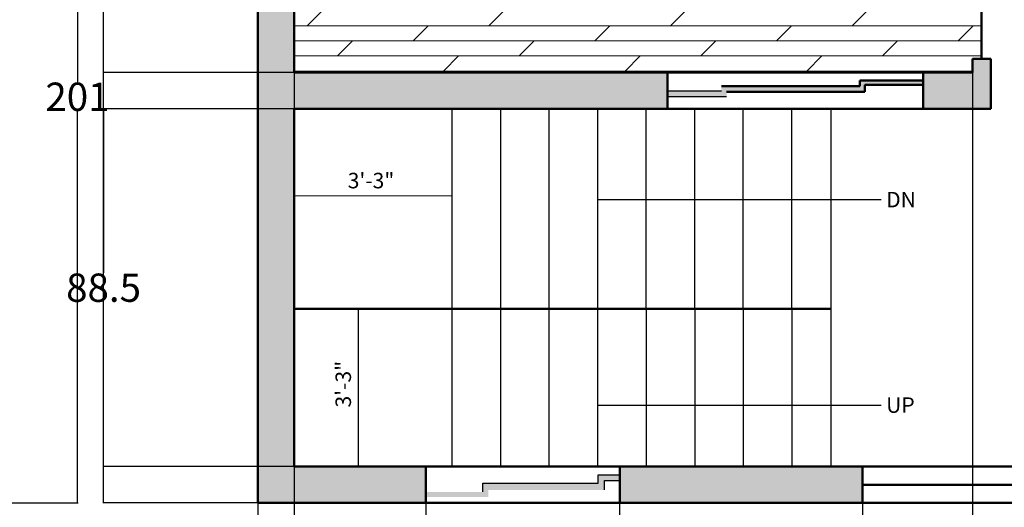
# Model space of a CAD drawing. Units: inches. Extents: x 1381 to 2246, y 1317 to 2168.
# Tile 10 of 15: x 1804 to 2048, y 1471 to 1591. Entities that reach past the tile are written whole.
import ezdxf

# ---------------------------------------------------------------- set-up
doc = ezdxf.new("R2010")
doc.units = ezdxf.units.IN
doc.header["$MEASUREMENT"] = 0
for name, color, linetype, lineweight in [('A-ANNO-DIMS', 2, 'Continuous', 18), ('A-ANNO-TEXT', 7, 'Continuous', 18), ('A-FLOR-PATT', 252, 'Continuous', 13), ('A-FLOR-STRS', 3, 'Continuous', 25), ('A-GLAZ', 4, 'Continuous', 25), ('A-WALL', 7, 'Continuous', 50), ('A-WALL-PATT', 8, 'Continuous', 13)]:
    doc.layers.add(name, color=color, linetype=linetype, lineweight=lineweight)
doc.styles.get("Standard").update_dxf_attribs({"font": 'arial.ttf'})
doc.dimstyles.get("Standard").update_dxf_attribs({"dimtxt": 7, "dimasz": 0.18, "dimexe": 0.18, "dimexo": 0.0625, "dimgap": 0.09, "dimtad": 0, "dimtih": 1, "dimtoh": 1, "dimdec": 1, "dimzin": 0, "dimdsep": 46, "dimlunit": 3, "dimtxsty": 'Standard', "dimcen": 0.09, "dimadec": 0, "dimazin": 0, "dimtfac": 1, "dimtdec": 1, "dimtofl": 0, "dimtmove": 0, "dimatfit": 3, "dimfxl": 1, "dimtolj": 1, "dimtzin": 0, "dimarcsym": 0})

# ---------------------------------------------------------------- blocks, each defined once
blk = doc.blocks.new('*D60')
at = {"layer": 'A-ANNO-DIMS', "color": 0, "lineweight": -2, "transparency": 16777216}
for p, q in [((1737.61, 1672.92), (1818.27, 1672.92)), ((1818.09, 1672.74), (1818.09, 1576.08)), ((1818.09, 1472.1), (1818.09, 1568.75)), ((1737.61, 1471.92), (1818.27, 1471.92))]:
    blk.add_line(p, q, dxfattribs=at)
at = {"layer": 'A-ANNO-DIMS', "color": 0, "transparency": 16777216}
for points in [[(1818.06, 1672.74), (1818.12, 1672.74), (1818.09, 1672.92)], [(1818.06, 1472.1), (1818.12, 1472.1), (1818.09, 1471.92)]]:
    blk.add_solid(points, dxfattribs=at)
at = {"layer": 'Defpoints', "color": 0, "transparency": 16777216}
for p in [(1737.55, 1672.92), (1818.09, 1672.92), (1737.55, 1471.92)]:
    blk.add_point(p, dxfattribs=at)
at = {"layer": 'A-ANNO-DIMS', "color": 0, "transparency": 16777216, "insert": (1818.09, 1572.42), "char_height": 7, "attachment_point": 5}
blk.add_mtext('\\A1;201', dxfattribs=at)
blk = doc.blocks.new('*D75')
at = {"layer": 'A-ANNO-DIMS', "color": 0, "lineweight": -2, "transparency": 16777216}
for p, q in [((1862.81, 1471.85), (1862.81, 1384.36)), ((2162.31, 1471.85), (2162.31, 1384.36)), ((1862.99, 1384.54), (2000.57, 1384.54)), ((2162.13, 1384.54), (2024.54, 1384.54))]:
    blk.add_line(p, q, dxfattribs=at)
at = {"layer": 'A-ANNO-DIMS', "color": 0, "transparency": 16777216}
for points in [[(1862.99, 1384.57), (1862.99, 1384.51), (1862.81, 1384.54)], [(2162.13, 1384.57), (2162.13, 1384.51), (2162.31, 1384.54)]]:
    blk.add_solid(points, dxfattribs=at)
at = {"layer": 'Defpoints', "color": 0, "transparency": 16777216}
for p in [(1862.81, 1471.92), (2162.31, 1471.92), (2162.31, 1384.54)]:
    blk.add_point(p, dxfattribs=at)
at = {"layer": 'A-ANNO-DIMS', "color": 0, "transparency": 16777216, "insert": (2012.56, 1384.54), "char_height": 7, "attachment_point": 5}
blk.add_mtext('\\A1;299.5', dxfattribs=at)
blk = doc.blocks.new('*D76')
at = {"layer": 'A-ANNO-DIMS', "color": 0, "lineweight": -2, "transparency": 16777216}
for p, q in [((1862.74, 2092.92), (1824.38, 2092.92)), ((1824.56, 2092.74), (1824.56, 1786.08)), ((1824.56, 1472.1), (1824.56, 1778.75)), ((1862.74, 1471.92), (1824.38, 1471.92))]:
    blk.add_line(p, q, dxfattribs=at)
at = {"layer": 'A-ANNO-DIMS', "color": 0, "transparency": 16777216}
for points in [[(1824.53, 2092.74), (1824.59, 2092.74), (1824.56, 2092.92)], [(1824.53, 1472.1), (1824.59, 1472.1), (1824.56, 1471.92)]]:
    blk.add_solid(points, dxfattribs=at)
at = {"layer": 'Defpoints', "color": 0, "transparency": 16777216}
for p in [(1824.56, 2092.92), (1862.81, 2092.92), (1862.81, 1471.92)]:
    blk.add_point(p, dxfattribs=at)
at = {"layer": 'A-ANNO-DIMS', "color": 0, "transparency": 16777216, "insert": (1824.56, 1782.42), "char_height": 7, "attachment_point": 5}
blk.add_mtext('\\A1;621', dxfattribs=at)
blk = doc.blocks.new('*D80')
at = {"layer": 'A-ANNO-DIMS', "color": 0, "lineweight": -2, "transparency": 16777216}
for p, q in [((1871.74, 1569.42), (1824.38, 1569.42)), ((1824.56, 1569.24), (1824.56, 1528.83)), ((1824.56, 1481.1), (1824.56, 1521.5)), ((1871.74, 1480.92), (1824.38, 1480.92))]:
    blk.add_line(p, q, dxfattribs=at)
at = {"layer": 'A-ANNO-DIMS', "color": 0, "transparency": 16777216}
for points in [[(1824.53, 1569.24), (1824.59, 1569.24), (1824.56, 1569.42)], [(1824.53, 1481.1), (1824.59, 1481.1), (1824.56, 1480.92)]]:
    blk.add_solid(points, dxfattribs=at)
at = {"layer": 'Defpoints', "color": 0, "transparency": 16777216}
for p in [(1824.56, 1569.42), (1871.81, 1569.42), (1871.81, 1480.92)]:
    blk.add_point(p, dxfattribs=at)
at = {"layer": 'A-ANNO-DIMS', "color": 0, "transparency": 16777216, "insert": (1824.56, 1525.17), "char_height": 7, "attachment_point": 5}
blk.add_mtext('\\A1;88.5', dxfattribs=at)
blk = doc.blocks.new('*D81')
at = {"layer": 'A-ANNO-DIMS', "color": 0, "lineweight": -2, "transparency": 16777216}
for p, q in [((1871.74, 1710.42), (1824.38, 1710.42)), ((1824.56, 1710.24), (1824.56, 1648.08)), ((1824.56, 1578.6), (1824.56, 1640.75)), ((1871.74, 1578.42), (1824.38, 1578.42))]:
    blk.add_line(p, q, dxfattribs=at)
at = {"layer": 'A-ANNO-DIMS', "color": 0, "transparency": 16777216}
for points in [[(1824.53, 1710.24), (1824.59, 1710.24), (1824.56, 1710.42)], [(1824.53, 1578.6), (1824.59, 1578.6), (1824.56, 1578.42)]]:
    blk.add_solid(points, dxfattribs=at)
at = {"layer": 'Defpoints', "color": 0, "transparency": 16777216}
for p in [(1824.56, 1710.42), (1871.81, 1710.42), (1871.81, 1578.42)]:
    blk.add_point(p, dxfattribs=at)
at = {"layer": 'A-ANNO-DIMS', "color": 0, "transparency": 16777216, "insert": (1824.56, 1644.42), "char_height": 7, "attachment_point": 5}
blk.add_mtext('\\A1;132', dxfattribs=at)
blk = doc.blocks.new('*D88')
at = {"layer": 'A-ANNO-DIMS', "color": 0, "lineweight": -2, "transparency": 16777216}
for p, q in [((1862.81, 1471.85), (1862.81, 1384.36)), ((1904.42, 1471.85), (1904.42, 1384.36)), ((1862.99, 1384.54), (1872.25, 1384.54)), ((1904.24, 1384.54), (1894.98, 1384.54))]:
    blk.add_line(p, q, dxfattribs=at)
at = {"layer": 'A-ANNO-DIMS', "color": 0, "transparency": 16777216}
for points in [[(1862.99, 1384.57), (1862.99, 1384.51), (1862.81, 1384.54)], [(1904.24, 1384.57), (1904.24, 1384.51), (1904.42, 1384.54)]]:
    blk.add_solid(points, dxfattribs=at)
at = {"layer": 'Defpoints', "color": 0, "transparency": 16777216}
for p in [(1862.81, 1471.92), (1904.42, 1471.92), (1904.42, 1384.54)]:
    blk.add_point(p, dxfattribs=at)
at = {"layer": 'A-ANNO-DIMS', "color": 0, "transparency": 16777216, "insert": (1883.61, 1384.54), "char_height": 7, "attachment_point": 5}
blk.add_mtext('\\A1;41.61', dxfattribs=at)
blk = doc.blocks.new('*D89')
at = {"layer": 'A-ANNO-DIMS', "color": 0, "lineweight": -2, "transparency": 16777216}
for p, q in [((1904.42, 1471.85), (1904.42, 1384.36)), ((1952.4, 1471.85), (1952.4, 1384.36)), ((1904.6, 1384.54), (1916.36, 1384.54)), ((1952.22, 1384.54), (1940.46, 1384.54))]:
    blk.add_line(p, q, dxfattribs=at)
at = {"layer": 'A-ANNO-DIMS', "color": 0, "transparency": 16777216}
for points in [[(1904.6, 1384.57), (1904.6, 1384.51), (1904.42, 1384.54)], [(1952.22, 1384.57), (1952.22, 1384.51), (1952.4, 1384.54)]]:
    blk.add_solid(points, dxfattribs=at)
at = {"layer": 'Defpoints', "color": 0, "transparency": 16777216}
for p in [(1904.42, 1471.92), (1952.4, 1471.92), (1952.4, 1384.54)]:
    blk.add_point(p, dxfattribs=at)
at = {"layer": 'A-ANNO-DIMS', "color": 0, "transparency": 16777216, "insert": (1928.41, 1384.54), "char_height": 7, "attachment_point": 5}
blk.add_mtext('\\A1;47.98', dxfattribs=at)
blk = doc.blocks.new('*D90')
at = {"layer": 'A-ANNO-DIMS', "color": 0, "lineweight": -2, "transparency": 16777216}
for p, q in [((1952.4, 1471.85), (1952.4, 1384.36)), ((2012.56, 1471.85), (2012.56, 1384.36)), ((1952.58, 1384.54), (1970.53, 1384.54)), ((2012.38, 1384.54), (1994.42, 1384.54))]:
    blk.add_line(p, q, dxfattribs=at)
at = {"layer": 'A-ANNO-DIMS', "color": 0, "transparency": 16777216}
for points in [[(1952.58, 1384.57), (1952.58, 1384.51), (1952.4, 1384.54)], [(2012.38, 1384.57), (2012.38, 1384.51), (2012.56, 1384.54)]]:
    blk.add_solid(points, dxfattribs=at)
at = {"layer": 'Defpoints', "color": 0, "transparency": 16777216}
for p in [(1952.4, 1471.92), (2012.56, 1471.92), (2012.56, 1384.54)]:
    blk.add_point(p, dxfattribs=at)
at = {"layer": 'A-ANNO-DIMS', "color": 0, "transparency": 16777216, "insert": (1982.48, 1384.54), "char_height": 7, "attachment_point": 5}
blk.add_mtext('\\A1;60.15', dxfattribs=at)
blk = doc.blocks.new('*D91')
at = {"layer": 'A-ANNO-DIMS', "color": 0, "lineweight": -2, "transparency": 16777216}
for p, q in [((2012.56, 1471.85), (2012.56, 1384.36)), ((2153.31, 1471.85), (2153.31, 1384.36)), ((2012.74, 1384.54), (2068.61, 1384.54)), ((2153.13, 1384.54), (2097.25, 1384.54))]:
    blk.add_line(p, q, dxfattribs=at)
at = {"layer": 'A-ANNO-DIMS', "color": 0, "transparency": 16777216}
for points in [[(2012.74, 1384.57), (2012.74, 1384.51), (2012.56, 1384.54)], [(2153.13, 1384.57), (2153.13, 1384.51), (2153.31, 1384.54)]]:
    blk.add_solid(points, dxfattribs=at)
at = {"layer": 'Defpoints', "color": 0, "transparency": 16777216}
for p in [(2012.56, 1471.92), (2153.31, 1471.92), (2153.31, 1384.54)]:
    blk.add_point(p, dxfattribs=at)
at = {"layer": 'A-ANNO-DIMS', "color": 0, "transparency": 16777216, "insert": (2082.93, 1384.54), "char_height": 7, "attachment_point": 5}
blk.add_mtext('\\A1;140.75', dxfattribs=at)
blk = doc.blocks.new('*D92')
at = {"layer": 'A-ANNO-DIMS', "color": 0, "lineweight": -2, "transparency": 16777216}
for p, q in [((1871.81, 1578.35), (1871.81, 1384.36)), ((2039.81, 1578.35), (2039.81, 1384.36)), ((1871.99, 1384.54), (1948.3, 1384.54)), ((2039.63, 1384.54), (1963.31, 1384.54))]:
    blk.add_line(p, q, dxfattribs=at)
at = {"layer": 'A-ANNO-DIMS', "color": 0, "transparency": 16777216}
for points in [[(1871.99, 1384.57), (1871.99, 1384.51), (1871.81, 1384.54)], [(2039.63, 1384.57), (2039.63, 1384.51), (2039.81, 1384.54)]]:
    blk.add_solid(points, dxfattribs=at)
at = {"layer": 'Defpoints', "color": 0, "transparency": 16777216}
for p in [(1871.81, 1578.42), (2039.81, 1578.42), (2039.81, 1384.54)]:
    blk.add_point(p, dxfattribs=at)
at = {"layer": 'A-ANNO-DIMS', "color": 0, "transparency": 16777216, "insert": (1955.81, 1384.54), "char_height": 7, "attachment_point": 5}
blk.add_mtext('\\A1;168', dxfattribs=at)

msp = doc.modelspace()

# ---------------------------------------------------------------- hatches: boundary and pattern name
at = {"layer": 'A-FLOR-PATT'}
h = msp.add_hatch(dxfattribs=at)
h.set_pattern_fill('DOLMIT', color=256, scale=15)
h.paths.add_polyline_path([(2039.8052, 1710.4163), (2024.8052, 1710.4163), (1932.7523, 1710.4163), (1932.7523, 1683.9148), (1871.8052, 1683.9148), (1871.8052, 1578.4163), (2039.8052, 1578.4163), (2039.8052, 1581.7679), (2042.0552, 1581.7679), (2042.0552, 1618.2205), (2039.8052, 1618.2205)])
edge = h.paths.add_edge_path(flags=16)
edge.add_spline(control_points=[(1941.6512, 1599.2474), (1941.7034, 1599.1739), (1941.8185, 1599.0119), (1941.6311, 1598.7103), (1941.372, 1598.3387), (1941.6312, 1598.1308), (1941.7624, 1598.0254)], knot_values=[0, 0, 0, 0, 0.37399428, 0.82431366, 1.46117297, 2.11445126, 2.11445126, 2.11445126, 2.11445126], degree=3, periodic=0)
edge.add_spline(control_points=[(1941.9859, 1599.2474), (1942.0381, 1599.1739), (1942.1532, 1599.0119), (1941.9659, 1598.7103), (1941.7067, 1598.3387), (1941.9659, 1598.1308), (1942.0971, 1598.0254)], knot_values=[0, 0, 0, 0, 0.37399428, 0.82431366, 1.46117297, 2.11445126, 2.11445126, 2.11445126, 2.11445126], degree=3, periodic=0)
edge = h.paths.add_edge_path(flags=16)
edge.add_line((1944.1282, 1667.7293), (1944.1282, 1599.2474))
edge.add_line((1944.1282, 1599.2474), (1915.5728, 1599.2474))
edge.add_line((1915.5728, 1599.2474), (1915.5728, 1606.0382))
edge.add_line((1915.5728, 1606.0382), (1889.4451, 1606.0382))
edge.add_line((1889.4451, 1606.0382), (1889.5561, 1594.5315))
edge.add_line((1889.5561, 1594.5315), (1876.3603, 1594.5315))
edge.add_line((1876.3603, 1594.5315), (1876.2493, 1606.0382))
edge.add_line((1876.2493, 1606.0382), (1876.2493, 1657.3975))
edge.add_line((1876.2493, 1657.3975), (1876.1383, 1668.9042))
edge.add_line((1876.1383, 1668.9042), (1889.3342, 1668.9042))
edge.add_line((1889.3342, 1668.9042), (1889.4451, 1657.3975))
edge.add_line((1889.4451, 1657.3975), (1915.5728, 1657.3975))
edge.add_line((1915.5728, 1657.3975), (1915.5728, 1667.7293))
edge.add_line((1915.5728, 1667.7293), (1941.69, 1667.7293))
edge.add_spline(control_points=[(1941.69, 1667.7293), (1941.7379, 1667.7989), (1941.8471, 1667.9576), (1941.661, 1668.2542), (1941.4024, 1668.626), (1941.6615, 1668.8339), (1941.7927, 1668.9392)], knot_values=[0, 0, 0, 0, 0.3521435, 0.80246288, 1.43932219, 2.09260048, 2.09260048, 2.09260048, 2.09260048], degree=3, periodic=0)
edge.add_spline(control_points=[(1942.1275, 1668.9392), (1941.9963, 1668.8339), (1941.7372, 1668.626), (1941.9957, 1668.2542), (1942.1818, 1667.9576), (1942.0727, 1667.7989), (1942.0248, 1667.7293)], knot_values=[0, 0, 0, 0, 0.65327829, 1.2901376, 1.74045698, 2.09260048, 2.09260048, 2.09260048, 2.09260048], degree=3, periodic=0)
edge.add_line((1942.0248, 1667.7293), (1944.1282, 1667.7293))
h.paths.add_polyline_path([(1893.809, 1657.3422), (1893.809, 1648.0757), (1886.9767, 1648.0757), (1886.9307, 1648.0133), (1886.9307, 1611.8376), (1879.1699, 1611.8376), (1879.1699, 1626.8866), (1886.9307, 1626.8866), (1886.9307, 1633.0267), (1879.1699, 1633.0267), (1879.1699, 1648.0757), (1886.9767, 1648.0757)], flags=0)
h.paths.add_polyline_path([(1886.984, 1663.4608, -1), (1878.4885, 1663.4608, -1)], flags=0)
h.paths.add_polyline_path([(1887.0949, 1600.5947, -1), (1878.5995, 1600.5947, -1)], flags=0)
h.paths.add_polyline_path([(1963.1209, 1621.5603), (2032.2362, 1621.5603), (2032.2362, 1633.9282), (1963.1209, 1633.9282)], flags=24)
h.paths.add_polyline_path([(1966.4202, 1633.6986), (2028.882, 1633.6986), (2028.882, 1646.2317), (1966.4202, 1646.2317)], flags=24)
at = {"layer": 'A-GLAZ'}
h = msp.add_hatch(color=256, dxfattribs=at)
h.dxf.hatch_style = 1
h.paths.add_polyline_path([(1978.8724, 1573.662), (2013.1608, 1573.662), (2013.1608, 1575.3695), (2027.577, 1575.3695), (2027.577, 1576.4366), (2011.879, 1576.4366), (2011.879, 1575.0493), (1977.5905, 1575.0493), (1977.5905, 1573.9163), (1964.2348, 1573.9163), (1964.2348, 1572.4881), (1978.8724, 1572.4881)])
h = msp.add_hatch(color=256, dxfattribs=at)
h.dxf.hatch_style = 1
h.paths.add_polyline_path([(1919.8747, 1475.1168), (1948.6648, 1475.1168), (1948.6648, 1477.4669), (1952.401, 1477.4669), (1952.401, 1478.8247), (1947.0532, 1478.8247), (1947.0532, 1476.8141), (1918.4828, 1476.8141), (1918.4828, 1474.6468), (1904.4174, 1474.6468), (1904.4174, 1473.3412), (1919.8747, 1473.3412)])
at = {"layer": 'A-WALL-PATT'}
h = msp.add_hatch(color=256, dxfattribs=at)
h.dxf.hatch_style = 1
h.paths.add_polyline_path([(1990.4785, 1915.9163), (1929.807, 1915.9163), (1929.807, 1911.4163), (1990.4785, 1911.4163)], flags=17)
h.paths.add_polyline_path([(1900.7902, 1915.9163), (1871.8052, 1915.9163), (1871.8052, 1911.4163), (1900.7902, 1911.4163)], flags=17)
h.paths.add_polyline_path([(2043.2216, 1915.9163), (2038.3052, 1915.9163), (2038.3052, 2035.4163), (2098.0373, 2035.4163), (2098.0373, 2039.9163), (2033.8052, 2039.9163), (2033.8052, 1915.9163), (2028.7731, 1915.9163), (2028.7731, 1911.4163), (2043.2216, 1911.4163)], flags=17)
h.paths.add_polyline_path([(2153.3052, 1915.9163), (2085.2216, 1915.9163), (2085.2216, 1911.4163), (2153.3052, 1911.4163)], flags=17)
h.paths.add_polyline_path([(1935.508, 1911.4163), (1931.008, 1911.4163), (1931.008, 1779.4163), (1899.8394, 1779.4163), (1899.8394, 1774.9163), (1902.8052, 1774.9163), (1979.3052, 1774.9163), (1979.3052, 1770.3401), (1983.8052, 1770.3401), (1983.8052, 1779.4163), (1935.508, 1779.4163)], flags=17)
h.paths.add_polyline_path([(1871.8052, 2083.9163), (2153.3052, 2083.9163), (2153.3052, 2039.9163), (2141.7178, 2039.9163), (2141.7178, 2035.4163), (2153.3052, 2035.4163), (2153.3052, 1471.9163), (2162.3052, 1471.9163), (2162.3052, 2092.9163), (1862.8052, 2092.9163), (1862.8052, 1471.9163), (1904.4174, 1471.9163), (1904.4174, 1480.9163), (1871.8052, 1480.9163), (1871.8052, 1569.4163), (1964.2348, 1569.4163), (1964.2348, 1578.4163), (1871.8052, 1578.4163)])
h.paths.add_polyline_path([(1907.3052, 1729.193), (1902.8052, 1729.193), (1902.8052, 1714.9163), (1871.8052, 1714.9163), (1871.8052, 1710.4163), (1932.8736, 1710.4163), (1932.8736, 1714.9163), (1907.3052, 1714.9163)], flags=17)
h.paths.add_polyline_path([(2044.3052, 1644.4163), (2039.8052, 1644.4163), (2039.8052, 1618.2205), (2044.3052, 1618.2205)], flags=17)
h.paths.add_polyline_path([(2044.3052, 1581.7679), (2039.8052, 1581.7679), (2039.8052, 1578.4163), (2027.577, 1578.4163), (2027.577, 1569.4163), (2044.3052, 1569.4163)], flags=17)
h = msp.add_hatch(color=256, dxfattribs=at)
h.dxf.hatch_style = 1
h.paths.add_polyline_path([(1873.9195, 1779.4163), (1871.8052, 1779.4163), (1871.8052, 1774.9163), (1873.9195, 1774.9163)])
h.paths.add_polyline_path([(1983.8052, 1779.4163), (1935.508, 1779.4163), (1935.508, 1911.4163), (1931.008, 1911.4163), (1931.008, 1779.4163), (1899.8394, 1779.4163), (1899.8394, 1774.9163), (1902.8052, 1774.9163), (1979.3052, 1774.9163), (1979.3052, 1770.3401), (1983.8052, 1770.3401)])
h.paths.add_polyline_path([(1907.3052, 1774.9163), (1902.8052, 1774.9163), (1902.8052, 1755.1129), (1907.3052, 1755.1129)])
h.paths.add_polyline_path([(1983.8052, 1734.7997), (1979.3052, 1734.7997), (1979.3052, 1714.9163), (1973.3503, 1714.9163), (1973.3503, 1710.4163), (1983.8052, 1710.4163)])
h.paths.add_polyline_path([(2044.3052, 1732.454), (2039.8052, 1732.454), (2039.8052, 1716.0149), (2024.8052, 1716.0149), (2024.8052, 1710.4163), (2039.8052, 1710.4163), (2039.8052, 1644.4163), (2044.3052, 1644.4163)])
h.paths.add_polyline_path([(2056.2659, 1677.4163), (2044.3052, 1677.4163), (2044.3052, 1672.9163), (2056.2659, 1672.9163)])
h.paths.add_polyline_path([(2119.6192, 1677.4163), (2104.2659, 1677.4163), (2104.2659, 1672.9163), (2119.6192, 1672.9163)])
h.paths.add_polyline_path([(2012.5552, 1480.9163), (1952.401, 1480.9163), (1952.401, 1471.9163), (2012.5552, 1471.9163)])
h.paths.add_polyline_path([(1870.8149, 1834.6368), (1933.6567, 1834.6368), (1933.6567, 1847.0047), (1870.8149, 1847.0047)], flags=9)

# ---------------------------------------------------------------- linework, layer by layer
at = {"layer": 'A-ANNO-DIMS'}
msp.add_line((1871.8052, 1547.9259), (1910.8052, 1547.9259), dxfattribs=at)
at = {"layer": 'A-FLOR-STRS'}
for p, q in [((1910.8052, 1569.4163), (1910.8052, 1480.9163)), ((1922.8427, 1569.4163), (1922.8427, 1480.9163)), ((1934.8802, 1569.4163), (1934.8802, 1480.9163)), ((1946.9176, 1569.4163), (1946.9176, 1480.9163)), ((1958.9551, 1519.9163), (1958.9551, 1569.4163)), ((1970.9926, 1519.9163), (1970.9926, 1569.4163)), ((1983.0301, 1519.9163), (1983.0301, 1569.4163)), ((1995.0676, 1519.9163), (1995.0676, 1569.4163)), ((2004.7266, 1569.4163), (2004.7266, 1480.9163)), ((1946.9176, 1546.9736), (2001.0969, 1546.9736)), ((2001.0969, 1546.9736), (2017.156, 1546.9736)), ((1887.6701, 1480.9163), (1887.6701, 1519.9163)), ((1958.9551, 1519.9163), (1958.9551, 1480.9163)), ((1970.9926, 1519.9163), (1970.9926, 1480.9163)), ((1983.0301, 1519.9163), (1983.0301, 1480.9163)), ((1995.0676, 1519.9163), (1995.0676, 1480.9163)), ((1946.9176, 1496.1305), (2001.0969, 1496.1305)), ((2001.0969, 1496.1305), (2017.156, 1496.1305)), ((1952.401, 1480.9163), (1904.4174, 1480.9163))]:
    msp.add_line(p, q, dxfattribs=at)
at = {"layer": 'A-GLAZ'}
for p, q in [((1964.2348, 1573.9163), (1977.5905, 1573.9163)), ((1964.2348, 1572.4881), (1978.8724, 1572.4881)), ((1947.0532, 1476.8141), (1947.0532, 1478.8247)), ((1947.0532, 1478.8247), (1952.401, 1478.8247)), ((1918.4828, 1474.6468), (1918.4828, 1476.8141)), ((1918.4828, 1476.8141), (1947.0532, 1476.8141)), ((1948.6648, 1475.1168), (1948.6648, 1477.4669)), ((1948.6648, 1477.4669), (1952.401, 1477.4669))]:
    msp.add_line(p, q, dxfattribs=at)
at = {"layer": 'A-WALL'}
for p, q in [((1862.8052, 2092.9163), (1862.8052, 1471.9163)), ((1871.8052, 2083.9163), (1871.8052, 1578.4163)), ((2042.0552, 1618.2205), (2042.0552, 1581.7679)), ((2039.8052, 1581.7679), (2044.3052, 1581.7679)), ((2039.8052, 1581.7679), (2039.8052, 1578.4163)), ((2044.3052, 1581.7679), (2044.3052, 1569.4163)), ((1871.8052, 1578.4163), (2039.8052, 1578.4163)), ((1964.2348, 1578.4163), (1964.2348, 1569.4163)), ((1964.2348, 1578.4163), (2027.577, 1578.4163)), ((2027.577, 1569.4163), (2027.577, 1578.4163)), ((2011.879, 1575.0493), (2011.879, 1576.4366)), ((2011.879, 1576.4366), (2027.577, 1576.4366)), ((1977.5905, 1575.0493), (2011.879, 1575.0493)), ((1978.8724, 1573.662), (2013.1608, 1573.662)), ((2013.1608, 1573.662), (2013.1608, 1575.3695)), ((2013.1608, 1575.3695), (2027.577, 1575.3695)), ((1871.8052, 1569.4163), (2044.3052, 1569.4163)), ((1871.8052, 1569.4163), (1871.8052, 1480.9163)), ((1964.2348, 1569.4163), (2027.577, 1569.4163)), ((1887.6701, 1519.9163), (1871.8052, 1519.9163)), ((1871.8052, 1519.9163), (2004.7266, 1519.9163)), ((1871.8052, 1480.9163), (2153.3052, 1480.9163)), ((1904.4174, 1480.9163), (1904.4174, 1471.9163)), ((1904.4174, 1480.9163), (1904.4174, 1474.6468)), ((1952.401, 1471.9163), (1952.401, 1480.9163)), ((2012.5552, 1480.9163), (2012.5552, 1471.9163)), ((2012.5552, 1480.9163), (2153.3052, 1480.9163)), ((2012.5552, 1471.9163), (2012.5552, 1480.9163)), ((2012.5552, 1480.9163), (2012.5552, 1476.4163)), ((2012.5552, 1476.4163), (2153.3052, 1476.4163)), ((1862.8052, 1471.9163), (2162.3052, 1471.9163)), ((1904.4174, 1471.9163), (1952.401, 1471.9163)), ((2153.3052, 1471.9163), (2012.5552, 1471.9163))]:
    msp.add_line(p, q, dxfattribs=at)

# ---------------------------------------------------------------- texts
at = {"layer": 'A-ANNO-TEXT'}
for s, p in [('3\'-3"', (1885.0325, 1549.7601)), ('DN', (2018.41, 1545.0483)), ('UP', (2018.41, 1494.2051))]:
    msp.add_text(s, height=3.83139, dxfattribs=at).set_placement(p)
msp.add_text('3\'-3"', height=3.83139, rotation=90, dxfattribs=at).set_placement((1885.8471, 1495.5207))

# ---------------------------------------------------------------- dimensions: what is measured, and where the dimension line sits
at = {"layer": 'A-ANNO-DIMS'}
for base, p1, p2, override, picture, middle in [((1824.5552, 2092.9163), (1862.8052, 1471.9163), (1862.8052, 2092.9163), {"dimdec": 0, "dimlfac": 1, "dimrnd": 0, "dimzin": 0, "dimdsep": 46, "dimlunit": 2}, '*D76', (1824.5552, 1782.4163)), ((1824.5552, 1710.4163), (1871.8052, 1578.4163), (1871.8052, 1710.4163), {"dimdec": 0, "dimlfac": 1, "dimrnd": 0, "dimzin": 0, "dimdsep": 46, "dimlunit": 2}, '*D81', (1824.5552, 1644.4163)), ((1818.0904, 1672.9163), (1737.551, 1471.9163), (1737.551, 1672.9163), {"dimdec": 0, "dimlfac": 1, "dimrnd": 0, "dimzin": 0, "dimdsep": 46, "dimlunit": 2}, '*D60', (1818.0904, 1572.4163)), ((1824.5552, 1569.4163), (1871.8052, 1480.9163), (1871.8052, 1569.4163), {"dimdec": 1, "dimlfac": 1, "dimrnd": 0, "dimzin": 0, "dimdsep": 46, "dimlunit": 2}, '*D80', (1824.5552, 1525.1663))]:
    dim = msp.add_linear_dim(base=base, p1=p1, p2=p2, angle=90, dimstyle='Standard', override=override, dxfattribs=at)
    dim.commit()
    dim.dimension.update_dxf_attribs({"geometry": picture, "text_midpoint": middle})
for base, p1, p2, override, picture, middle in [((2039.8052, 1384.5407), (1871.8052, 1578.4163), (2039.8052, 1578.4163), {"dimdec": 0, "dimlfac": 1, "dimrnd": 0, "dimzin": 0, "dimdsep": 46, "dimlunit": 2}, '*D92', (1955.8052, 1384.5407)), ((2162.3052, 1384.5407), (1862.8052, 1471.9163), (2162.3052, 1471.9163), {"dimdec": 1, "dimlfac": 1, "dimrnd": 0, "dimzin": 0, "dimdsep": 46, "dimlunit": 2}, '*D75', (2012.5552, 1384.5407)), ((1904.4174, 1384.5407), (1862.8052, 1471.9163), (1904.4174, 1471.9163), {"dimdec": 2, "dimlfac": 1, "dimrnd": 0, "dimzin": 0, "dimdsep": 46, "dimlunit": 2}, '*D88', (1883.6113, 1384.5407)), ((1952.401, 1384.5407), (1904.4174, 1471.9163), (1952.401, 1471.9163), {"dimdec": 2, "dimlfac": 1, "dimrnd": 0, "dimzin": 0, "dimdsep": 46, "dimlunit": 2}, '*D89', (1928.4092, 1384.5407)), ((2012.5552, 1384.5407), (1952.401, 1471.9163), (2012.5552, 1471.9163), {"dimdec": 2, "dimlfac": 1, "dimrnd": 0, "dimzin": 0, "dimdsep": 46, "dimlunit": 2}, '*D90', (1982.4781, 1384.5407)), ((2153.3052, 1384.5407), (2012.5552, 1471.9163), (2153.3052, 1471.9163), {"dimdec": 2, "dimlfac": 1, "dimrnd": 0, "dimzin": 0, "dimdsep": 46, "dimlunit": 2}, '*D91', (2082.9302, 1384.5407))]:
    dim = msp.add_linear_dim(base=base, p1=p1, p2=p2, dimstyle='Standard', override=override, dxfattribs=at)
    dim.commit()
    dim.dimension.update_dxf_attribs({"geometry": picture, "text_midpoint": middle})

doc.saveas('drawing.dxf')
